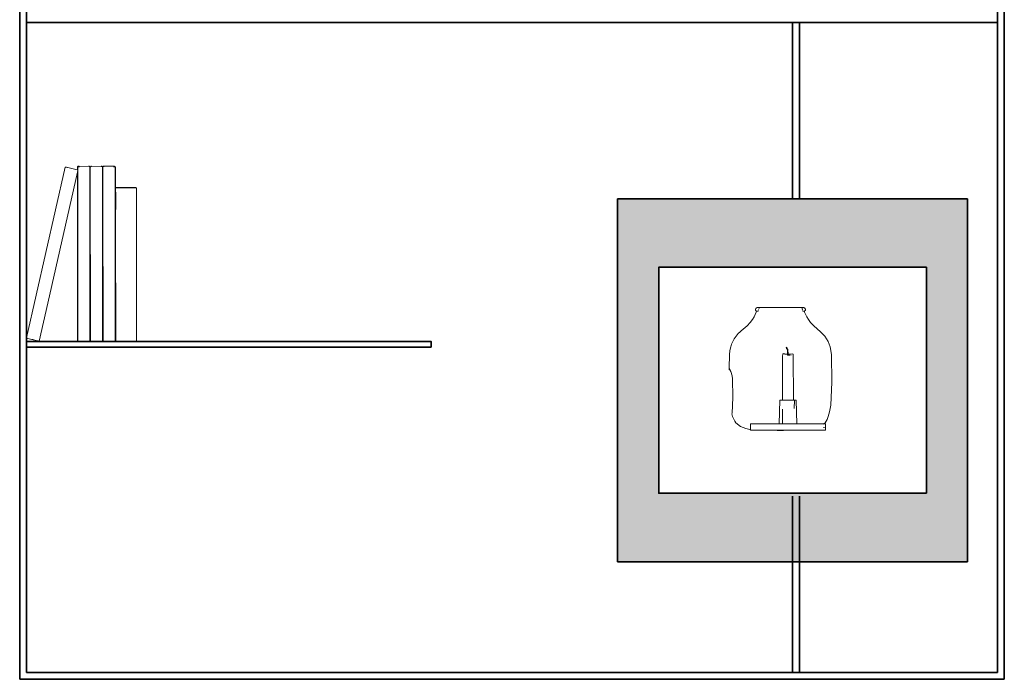
# Model space of a CAD drawing. Units: millimetres. Extents: x 2322 to 2394, y 1600 to 1790.
# Tile 1 of 5: x 2322 to 2394, y 1600 to 1648. Entities that reach past the tile are written whole.
import ezdxf

# ---------------------------------------------------------------- set-up
doc = ezdxf.new("R2010")
doc.units = ezdxf.units.MM
for name, color, linetype, lineweight in [('A-FURN', 7, 'Continuous', 35), ('A-FURN-ACCS', 8, 'Continuous', 18), ('A-FURN-PATT', 18, 'Continuous', 13)]:
    doc.layers.add(name, color=color, linetype=linetype, lineweight=lineweight)

msp = doc.modelspace()

# ---------------------------------------------------------------- hatches: boundary and pattern name
at = {"layer": 'A-FURN-PATT'}
h = msp.add_hatch(color=256, dxfattribs=at)
h.dxf.hatch_style = 1
h.paths.add_polyline_path([(2392.874, 1742.691), (2367.299, 1742.691), (2367.299, 1716.15), (2378.094, 1716.15), (2378.094, 1721.15), (2376.822, 1721.15), (2370.299, 1721.15), (2370.299, 1737.691), (2389.874, 1737.691), (2389.874, 1721.15), (2378.594, 1721.15), (2378.594, 1716.15), (2392.874, 1716.15)])
h.paths.add_polyline_path([(2352.154, 1685.571), (2339.867, 1685.571), (2339.867, 1680.571), (2349.154, 1680.571), (2349.154, 1664.029), (2329.579, 1664.029), (2329.579, 1680.571), (2339.367, 1680.571), (2339.367, 1685.571), (2326.579, 1685.571), (2326.579, 1659.029), (2352.154, 1659.029)])
h.paths.add_polyline_path([(2390.882, 1635.073), (2365.307, 1635.073), (2365.307, 1608.531), (2390.882, 1608.531)])
h.paths.add_polyline_path([(2387.882, 1630.073), (2387.882, 1613.531), (2368.307, 1613.531), (2368.307, 1630.073)], flags=16)
h.paths.add_polyline_path([(2373.463, 1622.711), (2373.46, 1622.644), (2373.462, 1622.642)], flags=0)
h.paths.add_polyline_path([(2380.387, 1618.619), (2380.387, 1618.619), (2380.35, 1618.619)], flags=0)
h.paths.add_polyline_path([(2377.431, 1618.132), (2377.363, 1618.141), (2377.19, 1618.152), (2377.145, 1618.149), (2376.982, 1618.132)], flags=0)
h.paths.add_polyline_path([(2376.126, 1618.152), (2375.767, 1618.152), (2375.734, 1618.152), (2375.734, 1618.152), (2375.028, 1618.152), (2375.028, 1618.198), (2374.578, 1618.295), (2374.235, 1618.449), (2373.926, 1618.69), (2373.709, 1619.163), (2373.66, 1619.336), (2373.672, 1619.402), (2373.73, 1620.54), (2373.702, 1622.038), (2373.678, 1622.131), (2373.705, 1621.917), (2373.73, 1620.54), (2373.667, 1619.311), (2373.709, 1619.163), (2373.87, 1618.812), (2373.949, 1618.699), (2374.037, 1618.604), (2374.187, 1618.486), (2374.3, 1618.42), (2374.485, 1618.337), (2374.688, 1618.272), (2374.979, 1618.209), (2375.028, 1618.203), (2375.028, 1618.372), (2375.028, 1618.619), (2377.125, 1618.619), (2377.165, 1620.356), (2377.172, 1620.356), (2377.172, 1620.357), (2377.341, 1620.357), (2377.354, 1620.357), (2377.354, 1623.532), (2377.38, 1623.766), (2377.629, 1623.72), (2377.726, 1623.72), (2377.722, 1623.891), (2377.719, 1624.041), (2377.644, 1624.123), (2377.631, 1624.228), (2377.644, 1624.211), (2377.677, 1624.213), (2377.688, 1624.153), (2377.757, 1624.059), (2377.78, 1623.72), (2377.883, 1623.72), (2378.152, 1623.76), (2378.155, 1620.358), (2378.298, 1620.356), (2378.301, 1620.356), (2378.362, 1620.357), (2378.402, 1618.619), (2377.354, 1618.619), (2377.125, 1618.619), (2375.028, 1618.619), (2375.028, 1618.372), (2375.028, 1618.177), (2375.049, 1618.152), (2375.734, 1618.152), (2375.756, 1618.153), (2375.767, 1618.152), (2376.126, 1618.152), (2376.144, 1618.154), (2376.168, 1618.151)], flags=0)
h.paths.add_polyline_path([(2380.5, 1618.343), (2380.401, 1618.342), (2380.5, 1618.342)], flags=0)
h.paths.add_polyline_path([(2378.836, 1627.111), (2378.86, 1627.114), (2378.771, 1627.114), (2378.773, 1627.108)], flags=0)
h.paths.add_polyline_path([(2378.972, 1627.091), (2379.09, 1626.957), (2378.972, 1626.879), (2378.964, 1626.862), (2378.975, 1626.787), (2379.128, 1626.434), (2379.25, 1626.246), (2379.42, 1626.03), (2379.646, 1625.791), (2380.15, 1625.354), (2380.519, 1624.956), (2380.743, 1624.553), (2380.884, 1624.119), (2380.94, 1623.673), (2380.977, 1621.652), (2380.892, 1619.98), (2380.807, 1619.502), (2380.712, 1619.163), (2380.621, 1618.942), (2380.422, 1618.619), (2380.413, 1618.619), (2380.386, 1618.619), (2380.474, 1618.703), (2380.621, 1618.942), (2380.712, 1619.163), (2380.807, 1619.502), (2380.892, 1619.98), (2380.977, 1621.652), (2380.94, 1623.673), (2380.9, 1623.987), (2380.843, 1624.244), (2380.778, 1624.446), (2380.693, 1624.644), (2380.585, 1624.839), (2380.452, 1625.029), (2380.15, 1625.354), (2379.646, 1625.791), (2379.324, 1626.132), (2379.128, 1626.434), (2378.92, 1626.915), (2378.841, 1626.975), (2378.869, 1626.811), (2379.027, 1626.915), (2379.041, 1626.939), (2379.037, 1626.997), (2379.02, 1627.036), (2378.879, 1627.196), (2378.841, 1627.151)], flags=0)
h.paths.add_polyline_path([(2375.501, 1627.114), (2375.642, 1627.103), (2375.561, 1626.855), (2375.555, 1626.827), (2375.48, 1626.868), (2375.292, 1626.434), (2375.097, 1626.132), (2374.775, 1625.791), (2374.271, 1625.354), (2374.13, 1625.216), (2373.969, 1625.029), (2373.836, 1624.839), (2373.728, 1624.644), (2373.643, 1624.446), (2373.537, 1624.119), (2373.52, 1623.987), (2373.601, 1624.348), (2373.773, 1624.748), (2374.034, 1625.122), (2374.271, 1625.354), (2374.775, 1625.791), (2375.001, 1626.03), (2375.171, 1626.246), (2375.292, 1626.434), (2375.445, 1626.787), (2375.447, 1626.797), (2375.334, 1627.042)], flags=0)
h.paths.add_polyline_path([(2375.398, 1627.114), (2375.384, 1626.997), (2375.411, 1627.054), (2375.531, 1627.169), (2375.597, 1627.114)], flags=0)
h.paths.add_polyline_path([(2377.985, 1623.628), (2377.785, 1623.645), (2377.786, 1623.634), (2377.764, 1623.634), (2377.729, 1623.636), (2377.728, 1623.656), (2377.701, 1623.664), (2377.421, 1623.752), (2377.412, 1623.748), (2377.629, 1623.72), (2377.78, 1623.72), (2377.783, 1623.68)], flags=0)
h.paths.add_polyline_path([(2377.348, 1620.356), (2377.335, 1620.356), (2377.327, 1620.356), (2377.354, 1620.356)], flags=0)
h.paths.add_polyline_path([(2377.834, 1620.357), (2377.854, 1620.356), (2377.911, 1620.356), (2377.923, 1620.357)], flags=0)
h.paths.add_polyline_path([(2378.155, 1620.356), (2378.155, 1620.356), (2378.014, 1620.356), (2378.002, 1620.357), (2377.96, 1620.356), (2377.956, 1620.356), (2377.923, 1620.357), (2378.111, 1620.357), (2378.119, 1620.356), (2378.144, 1620.356), (2378.163, 1620.357), (2378.163, 1620.357), (2378.157, 1620.357), (2378.149, 1620.356)], flags=0)
h.paths.add_polyline_path([(2377.609, 1620.357), (2377.623, 1620.356), (2377.653, 1620.357), (2377.738, 1620.356), (2377.743, 1620.357)], flags=0)
h.paths.add_polyline_path([(2380.479, 1618.152), (2380.406, 1618.152), (2380.313, 1618.151), (2380.107, 1618.152), (2380.104, 1618.152), (2380.108, 1618.151), (2379.961, 1618.152), (2379.793, 1618.152), (2377.32, 1618.152), (2377.3, 1618.149), (2377.253, 1618.152), (2379.793, 1618.152), (2380.01, 1618.153), (2380.21, 1618.152), (2380.229, 1618.152), (2380.231, 1618.152), (2380.394, 1618.152), (2380.48, 1618.152)], flags=0)

# ---------------------------------------------------------------- linework, layer by layer
at = {"layer": 'A-FURN'}
for p, q in [((2321.58, 1599.925), (2321.58, 1755.925)), ((2322.08, 1600.425), (2322.08, 1755.425)), ((2393.08, 1755.425), (2393.08, 1600.425)), ((2393.58, 1755.925), (2393.58, 1599.925)), ((2393.08, 1695.937), (2393.08, 1600.425)), ((2393.08, 1647.981), (2322.08, 1647.981)), ((2322.08, 1647.981), (2322.08, 1600.425)), ((2378.094, 1635.073), (2378.094, 1647.981)), ((2378.594, 1635.073), (2378.594, 1647.981)), ((2390.882, 1635.073), (2390.882, 1608.531)), ((2378.094, 1600.425), (2378.094, 1613.334)), ((2378.594, 1600.425), (2378.594, 1613.334)), ((2393.58, 1599.925), (2321.58, 1599.925)), ((2393.08, 1600.425), (2322.08, 1600.425))]:
    msp.add_line(p, q, dxfattribs=at)
for points in [[(2390.882, 1608.531), (2365.307, 1608.531), (2365.307, 1635.073), (2390.882, 1635.073)], [(2322.08, 1624.628), (2347.625, 1624.628), (2351.673, 1624.628), (2351.673, 1624.228)], [(2322.08, 1624.228), (2347.625, 1624.228), (2351.673, 1624.228)]]:
    msp.add_lwpolyline(points, dxfattribs=at)
msp.add_lwpolyline([(2387.882, 1613.531), (2368.307, 1613.531), (2368.307, 1630.073), (2387.882, 1630.073)], close=True, dxfattribs=at)
at = {"layer": 'A-FURN-ACCS'}
for p, q in [((2322.08, 1624.914), (2324.904, 1637.395)), ((2324.905, 1637.395), (2322.089, 1624.904)), ((2324.904, 1637.395), (2324.905, 1637.395)), ((2324.905, 1637.395), (2325.014, 1637.38)), ((2325.29, 1637.308), (2325.014, 1637.38)), ((2325.29, 1637.308), (2325.067, 1637.358)), ((2325.773, 1637.199), (2325.29, 1637.308)), ((2325.813, 1637.444), (2325.798, 1637.401)), ((2325.798, 1637.401), (2325.798, 1637.202)), ((2325.813, 1637.409), (2325.813, 1637.444)), ((2325.813, 1637.444), (2325.822, 1637.444)), ((2325.822, 1637.444), (2325.826, 1637.446)), ((2325.822, 1637.444), (2325.822, 1637.191)), ((2325.826, 1637.446), (2325.847, 1637.458)), ((2325.826, 1637.446), (2325.86, 1637.451)), ((2325.839, 1637.444), (2325.826, 1637.446)), ((2325.864, 1637.449), (2325.839, 1637.444)), ((2325.875, 1637.444), (2325.839, 1637.444)), ((2325.903, 1637.458), (2325.847, 1637.458)), ((2325.86, 1637.451), (2325.847, 1637.458)), ((2325.86, 1637.451), (2325.862, 1637.452)), ((2325.862, 1637.452), (2325.903, 1637.458)), ((2325.864, 1637.449), (2325.862, 1637.452)), ((2325.866, 1637.45), (2325.864, 1637.449)), ((2325.903, 1637.458), (2325.866, 1637.45)), ((2325.874, 1637.444), (2325.866, 1637.45)), ((2325.875, 1637.444), (2325.874, 1637.444)), ((2325.877, 1637.402), (2325.875, 1637.444)), ((2325.878, 1637.444), (2325.875, 1637.444)), ((2325.877, 1637.444), (2325.875, 1637.444)), ((2325.877, 1637.402), (2325.877, 1637.444)), ((2325.878, 1637.444), (2325.877, 1637.444)), ((2325.878, 1637.444), (2325.903, 1637.458)), ((2325.901, 1637.445), (2325.878, 1637.444)), ((2325.901, 1637.445), (2325.9, 1637.403)), ((2325.903, 1637.458), (2325.901, 1637.445)), ((2325.901, 1637.445), (2325.902, 1637.403)), ((2325.904, 1637.445), (2325.901, 1637.445)), ((2325.926, 1637.445), (2325.903, 1637.458)), ((2325.903, 1637.458), (2325.904, 1637.445)), ((2325.904, 1637.445), (2325.905, 1637.403)), ((2325.926, 1637.445), (2325.904, 1637.445)), ((2325.929, 1637.444), (2325.926, 1637.445)), ((2326.62, 1637.457), (2325.929, 1637.444)), ((2325.929, 1637.444), (2325.93, 1637.404)), ((2326.6, 1637.441), (2326.6, 1637.444)), ((2326.622, 1637.458), (2326.62, 1637.457)), ((2326.624, 1637.457), (2326.62, 1637.457)), ((2326.621, 1637.442), (2326.621, 1637.444)), ((2326.622, 1637.458), (2326.624, 1637.457)), ((2326.624, 1637.457), (2326.678, 1637.458)), ((2326.625, 1637.442), (2326.625, 1637.444)), ((2326.658, 1637.444), (2326.687, 1637.444)), ((2326.684, 1637.448), (2326.668, 1637.45)), ((2326.684, 1637.448), (2326.678, 1637.458)), ((2326.708, 1637.444), (2326.684, 1637.448)), ((2326.687, 1637.444), (2326.684, 1637.448)), ((2326.687, 1637.444), (2326.708, 1637.444)), ((2326.712, 1637.401), (2326.687, 1637.444)), ((2326.712, 1637.444), (2326.708, 1637.444)), ((2326.708, 1637.444), (2326.727, 1637.401)), ((2326.71, 1624.631), (2326.712, 1637.401)), ((2326.727, 1637.401), (2326.712, 1637.444)), ((2326.727, 1637.401), (2326.712, 1624.637)), ((2326.727, 1637.401), (2326.746, 1637.444)), ((2326.727, 1624.671), (2326.727, 1637.401)), ((2326.746, 1624.628), (2326.727, 1637.401)), ((2326.742, 1624.628), (2326.727, 1637.401)), ((2326.742, 1637.401), (2326.747, 1637.409)), ((2326.75, 1624.628), (2326.742, 1637.401)), ((2326.774, 1637.448), (2326.746, 1637.444)), ((2326.747, 1637.409), (2326.746, 1637.409)), ((2326.747, 1637.409), (2326.767, 1637.444)), ((2326.774, 1637.448), (2326.767, 1637.444)), ((2326.788, 1637.458), (2326.774, 1637.448)), ((2326.794, 1637.452), (2326.774, 1637.448)), ((2326.788, 1637.458), (2326.794, 1637.452)), ((2326.831, 1637.457), (2326.788, 1637.458)), ((2326.804, 1637.453), (2326.794, 1637.452)), ((2326.794, 1637.452), (2326.802, 1637.444)), ((2326.802, 1637.444), (2326.806, 1637.444)), ((2326.806, 1637.444), (2326.816, 1637.45)), ((2326.806, 1637.444), (2326.829, 1637.444)), ((2326.829, 1637.444), (2326.83, 1637.446)), ((2326.836, 1637.444), (2326.829, 1637.444)), ((2326.831, 1637.457), (2326.832, 1637.458)), ((2326.832, 1637.458), (2326.834, 1637.457)), ((2327.54, 1637.445), (2326.834, 1637.457)), ((2327.54, 1637.445), (2327.548, 1637.458)), ((2327.554, 1637.444), (2327.54, 1637.445)), ((2327.548, 1637.458), (2327.611, 1637.458)), ((2327.553, 1637.447), (2327.554, 1637.444)), ((2327.587, 1637.444), (2327.554, 1637.444)), ((2327.616, 1637.444), (2327.579, 1637.452)), ((2327.616, 1637.444), (2327.611, 1637.458)), ((2327.622, 1637.438), (2327.616, 1637.444)), ((2327.641, 1637.401), (2327.622, 1637.438)), ((2327.656, 1637.401), (2327.622, 1637.438)), ((2327.641, 1627.214), (2327.656, 1637.401)), ((2327.656, 1637.401), (2327.641, 1624.671)), ((2327.641, 1627.214), (2327.641, 1637.401)), ((2327.656, 1624.671), (2327.671, 1637.401)), ((2327.671, 1637.401), (2327.67, 1637.444)), ((2327.67, 1637.444), (2327.673, 1637.444)), ((2327.671, 1637.401), (2327.673, 1637.444)), ((2327.671, 1637.401), (2327.672, 1635.669)), ((2327.706, 1637.458), (2327.673, 1637.444)), ((2327.673, 1637.444), (2327.675, 1637.444)), ((2327.716, 1637.451), (2327.675, 1637.444)), ((2327.706, 1637.458), (2328.524, 1637.458)), ((2327.735, 1637.444), (2327.758, 1637.444)), ((2327.758, 1637.444), (2327.758, 1637.442)), ((2327.762, 1637.442), (2327.762, 1637.444)), ((2327.78, 1637.444), (2327.786, 1637.444)), ((2327.786, 1637.44), (2327.786, 1637.444)), ((2328.468, 1637.444), (2328.465, 1637.404)), ((2328.483, 1637.444), (2328.477, 1637.403)), ((2328.483, 1637.444), (2328.481, 1637.403)), ((2328.483, 1637.403), (2328.483, 1637.444)), ((2328.506, 1637.402), (2328.506, 1637.444)), ((2328.509, 1637.401), (2328.51, 1637.444)), ((2328.554, 1637.446), (2328.524, 1637.458)), ((2328.537, 1637.449), (2328.539, 1637.448)), ((2328.539, 1637.448), (2328.554, 1637.446)), ((2328.554, 1637.446), (2328.544, 1637.444)), ((2328.561, 1637.444), (2328.554, 1637.446)), ((2328.561, 1637.444), (2328.562, 1624.628)), ((2328.566, 1637.444), (2328.561, 1637.444)), ((2328.57, 1637.444), (2328.566, 1637.444)), ((2328.566, 1637.444), (2328.57, 1637.434)), ((2328.585, 1637.401), (2328.57, 1637.444)), ((2328.57, 1637.444), (2328.57, 1637.434)), ((2328.57, 1637.434), (2328.57, 1637.409)), ((2328.57, 1637.434), (2328.585, 1637.401)), ((2328.585, 1624.671), (2328.585, 1637.401)), ((2325.797, 1637.027), (2323.637, 1627.451)), ((2325.792, 1637.205), (2325.773, 1637.199)), ((2325.773, 1637.199), (2325.822, 1637.188)), ((2325.792, 1637.205), (2325.798, 1637.202)), ((2325.797, 1637.027), (2325.822, 1637.139)), ((2325.797, 1637.027), (2325.798, 1624.671)), ((2325.822, 1637.191), (2325.798, 1637.202)), ((2325.798, 1637.202), (2325.798, 1637.197)), ((2325.822, 1637.139), (2325.821, 1624.628)), ((2325.831, 1637.186), (2325.822, 1637.191)), ((2325.822, 1637.191), (2325.822, 1637.188)), ((2325.831, 1637.186), (2325.822, 1637.188)), ((2325.822, 1637.146), (2325.831, 1637.186)), ((2325.822, 1637.146), (2325.822, 1637.139)), ((2328.585, 1624.671), (2328.597, 1635.853)), ((2328.596, 1635.889), (2328.6, 1635.889)), ((2328.597, 1635.853), (2328.596, 1635.889)), ((2328.597, 1635.853), (2328.6, 1635.889)), ((2328.597, 1635.853), (2328.599, 1635.297)), ((2328.632, 1635.901), (2328.6, 1635.889)), ((2328.639, 1635.889), (2328.6, 1635.889)), ((2328.632, 1635.901), (2328.643, 1635.889)), ((2330.048, 1635.901), (2328.632, 1635.901)), ((2328.665, 1635.889), (2328.632, 1635.901)), ((2328.643, 1635.889), (2328.639, 1635.889)), ((2328.646, 1635.889), (2328.643, 1635.889)), ((2328.643, 1635.889), (2328.645, 1635.889)), ((2328.645, 1635.889), (2328.646, 1635.889)), ((2328.665, 1635.889), (2328.646, 1635.889)), ((2328.665, 1635.889), (2328.676, 1635.889)), ((2328.676, 1635.889), (2328.679, 1635.889)), ((2328.679, 1635.889), (2330.031, 1635.889)), ((2330.031, 1635.889), (2330.048, 1635.901)), ((2330.05, 1635.899), (2330.031, 1635.889)), ((2330.031, 1635.889), (2330.05, 1635.889)), ((2330.048, 1635.901), (2330.05, 1635.901)), ((2330.05, 1635.899), (2330.05, 1635.901)), ((2330.085, 1635.901), (2330.05, 1635.901)), ((2330.08, 1635.896), (2330.05, 1635.901)), ((2330.05, 1635.889), (2330.05, 1635.899)), ((2330.053, 1635.889), (2330.05, 1635.899)), ((2330.058, 1635.889), (2330.05, 1635.899)), ((2330.053, 1635.889), (2330.05, 1635.889)), ((2330.053, 1635.889), (2330.058, 1635.889)), ((2330.074, 1635.889), (2330.058, 1635.889)), ((2330.074, 1635.889), (2330.08, 1635.896)), ((2330.074, 1635.889), (2330.11, 1635.891)), ((2330.08, 1635.896), (2330.085, 1635.901)), ((2330.11, 1635.891), (2330.08, 1635.896)), ((2330.11, 1635.891), (2330.085, 1635.901)), ((2330.115, 1635.889), (2330.11, 1635.891)), ((2330.115, 1624.628), (2330.115, 1635.889)), ((2330.118, 1635.889), (2330.115, 1635.889)), ((2330.121, 1635.889), (2330.118, 1635.889)), ((2330.118, 1635.889), (2330.121, 1635.881)), ((2330.133, 1635.853), (2330.121, 1635.889)), ((2330.121, 1635.889), (2330.121, 1635.881)), ((2330.121, 1635.881), (2330.121, 1635.859)), ((2330.121, 1635.881), (2330.133, 1635.853)), ((2330.133, 1624.662), (2330.133, 1635.853)), ((2327.672, 1635.669), (2327.656, 1624.671)), ((2327.672, 1635.669), (2327.679, 1624.628)), ((2328.599, 1635.297), (2328.596, 1633.242)), ((2328.596, 1633.242), (2328.585, 1624.671)), ((2328.596, 1624.635), (2328.596, 1633.242)), ((2328.596, 1633.242), (2328.603, 1624.628)), ((2323.011, 1624.674), (2323.637, 1627.451)), ((2323.637, 1627.451), (2323.013, 1624.674)), ((2327.641, 1624.671), (2327.641, 1627.214)), ((2375.292, 1626.434), (2375.445, 1626.787)), ((2375.378, 1626.947), (2375.384, 1626.997)), ((2375.378, 1626.947), (2375.391, 1626.918)), ((2375.384, 1626.997), (2375.411, 1627.054)), ((2375.435, 1626.893), (2375.391, 1626.918)), ((2375.411, 1627.054), (2375.453, 1627.094)), ((2375.457, 1626.862), (2375.435, 1626.893)), ((2375.445, 1626.787), (2375.457, 1626.862)), ((2375.453, 1627.094), (2375.501, 1627.114)), ((2375.501, 1627.114), (2375.608, 1627.106)), ((2375.501, 1627.114), (2376.761, 1627.114)), ((2375.561, 1626.855), (2375.551, 1626.805)), ((2375.576, 1626.901), (2375.561, 1626.855)), ((2375.602, 1626.979), (2375.585, 1626.929)), ((2375.608, 1627.106), (2375.647, 1627.074)), ((2375.647, 1627.074), (2375.65, 1627.055)), ((2376.774, 1627.114), (2376.761, 1627.114)), ((2376.774, 1627.114), (2378.86, 1627.114)), ((2378.768, 1627.108), (2378.836, 1627.111)), ((2378.793, 1627.096), (2378.774, 1627.075)), ((2378.785, 1627.017), (2378.812, 1626.997)), ((2378.836, 1627.111), (2378.793, 1627.096)), ((2378.812, 1626.997), (2378.818, 1626.978)), ((2378.834, 1626.934), (2378.837, 1626.925)), ((2378.86, 1627.114), (2378.836, 1627.111)), ((2378.842, 1626.91), (2378.861, 1626.857)), ((2378.863, 1627.114), (2378.86, 1627.114)), ((2378.861, 1626.857), (2378.87, 1626.803)), ((2378.863, 1627.114), (2378.923, 1627.114)), ((2378.972, 1627.091), (2378.923, 1627.114)), ((2378.964, 1626.862), (2378.972, 1626.879)), ((2378.975, 1626.787), (2378.964, 1626.862)), ((2379.02, 1627.036), (2378.972, 1627.091)), ((2378.972, 1626.879), (2379.027, 1626.915)), ((2379.128, 1626.434), (2378.975, 1626.787)), ((2379.037, 1626.997), (2379.02, 1627.036)), ((2379.027, 1626.915), (2379.041, 1626.939)), ((2379.041, 1626.939), (2379.037, 1626.997)), ((2374.334, 1625.409), (2374.775, 1625.791)), ((2374.775, 1625.791), (2375.001, 1626.03)), ((2375.001, 1626.03), (2375.171, 1626.246)), ((2375.171, 1626.246), (2375.292, 1626.434)), ((2379.25, 1626.246), (2379.128, 1626.434)), ((2379.42, 1626.03), (2379.25, 1626.246)), ((2379.646, 1625.791), (2379.42, 1626.03)), ((2380.15, 1625.354), (2379.646, 1625.791)), ((2373.969, 1625.029), (2374.13, 1625.216)), ((2374.13, 1625.216), (2374.271, 1625.354)), ((2374.271, 1625.354), (2374.334, 1625.409)), ((2380.452, 1625.029), (2380.15, 1625.354)), ((2322.08, 1624.914), (2322.084, 1624.883)), ((2322.084, 1624.883), (2322.089, 1624.904)), ((2322.084, 1624.883), (2322.086, 1624.883)), ((2322.089, 1624.904), (2322.086, 1624.883)), ((2322.181, 1624.862), (2322.086, 1624.883)), ((2322.181, 1624.862), (2322.471, 1624.786)), ((2322.471, 1624.786), (2322.549, 1624.779)), ((2322.996, 1624.668), (2322.471, 1624.786)), ((2322.692, 1624.746), (2322.549, 1624.779)), ((2322.692, 1624.746), (2322.695, 1624.745)), ((2322.996, 1624.668), (2322.961, 1624.684)), ((2322.996, 1624.668), (2322.997, 1624.678)), ((2322.996, 1624.668), (2323.011, 1624.674)), ((2323.013, 1624.674), (2323.011, 1624.674)), ((2325.798, 1624.671), (2325.813, 1624.628)), ((2325.813, 1624.637), (2325.798, 1624.671)), ((2325.813, 1624.628), (2325.813, 1624.637)), ((2325.817, 1624.628), (2325.813, 1624.637)), ((2325.813, 1624.628), (2325.817, 1624.628)), ((2325.821, 1624.628), (2325.817, 1624.628)), ((2325.821, 1624.628), (2326.71, 1624.628)), ((2326.712, 1624.637), (2326.71, 1624.631)), ((2326.71, 1624.628), (2326.71, 1624.631)), ((2326.71, 1624.628), (2326.712, 1624.628)), ((2326.712, 1624.628), (2326.727, 1624.671)), ((2326.727, 1624.671), (2326.712, 1624.637)), ((2326.712, 1624.637), (2326.712, 1624.628)), ((2326.742, 1624.628), (2326.712, 1624.628)), ((2326.746, 1624.628), (2326.742, 1624.628)), ((2326.746, 1624.628), (2326.75, 1624.628)), ((2327.633, 1624.628), (2326.75, 1624.628)), ((2327.637, 1624.651), (2327.633, 1624.628)), ((2327.637, 1624.628), (2327.633, 1624.628)), ((2327.641, 1624.671), (2327.637, 1624.651)), ((2327.637, 1624.628), (2327.637, 1624.651)), ((2327.641, 1624.628), (2327.637, 1624.628)), ((2327.641, 1624.671), (2327.641, 1624.628)), ((2327.67, 1624.628), (2327.641, 1624.628)), ((2327.656, 1624.671), (2327.67, 1624.628)), ((2327.67, 1624.637), (2327.656, 1624.671)), ((2327.67, 1624.628), (2327.67, 1624.637)), ((2327.675, 1624.628), (2327.67, 1624.637)), ((2327.67, 1624.628), (2327.675, 1624.628)), ((2327.679, 1624.628), (2327.675, 1624.628)), ((2327.679, 1624.628), (2328.562, 1624.628)), ((2328.566, 1624.628), (2328.562, 1624.628)), ((2328.57, 1624.637), (2328.566, 1624.628)), ((2328.566, 1624.628), (2328.57, 1624.628)), ((2328.57, 1624.628), (2328.585, 1624.671)), ((2328.585, 1624.671), (2328.57, 1624.637)), ((2328.57, 1624.663), (2328.57, 1624.637)), ((2328.57, 1624.637), (2328.57, 1624.628)), ((2328.596, 1624.628), (2328.57, 1624.628)), ((2328.585, 1624.662), (2328.585, 1624.671)), ((2328.585, 1624.662), (2328.596, 1624.628)), ((2328.596, 1624.635), (2328.585, 1624.662)), ((2328.596, 1624.628), (2328.596, 1624.635)), ((2328.599, 1624.628), (2328.596, 1624.635)), ((2328.599, 1624.628), (2328.596, 1624.628)), ((2328.603, 1624.628), (2328.599, 1624.628)), ((2330.115, 1624.628), (2328.603, 1624.628)), ((2330.119, 1624.628), (2330.115, 1624.628)), ((2330.121, 1624.634), (2330.119, 1624.628)), ((2330.122, 1624.628), (2330.119, 1624.628)), ((2330.133, 1624.662), (2330.121, 1624.634)), ((2330.121, 1624.634), (2330.122, 1624.628)), ((2330.122, 1624.628), (2330.133, 1624.662)), ((2373.578, 1624.244), (2373.643, 1624.446)), ((2373.643, 1624.446), (2373.728, 1624.644)), ((2373.836, 1624.839), (2373.728, 1624.644)), ((2373.969, 1625.029), (2373.836, 1624.839)), ((2380.585, 1624.839), (2380.452, 1625.029)), ((2380.693, 1624.644), (2380.585, 1624.839)), ((2380.778, 1624.446), (2380.693, 1624.644)), ((2380.843, 1624.244), (2380.778, 1624.446)), ((2373.463, 1622.711), (2373.481, 1623.673)), ((2373.481, 1623.673), (2373.52, 1623.987)), ((2373.52, 1623.987), (2373.578, 1624.244)), ((2377.354, 1623.532), (2377.376, 1623.731)), ((2377.431, 1623.757), (2377.376, 1623.731)), ((2377.629, 1623.72), (2377.431, 1623.757)), ((2377.589, 1623.699), (2377.449, 1623.743)), ((2377.449, 1623.743), (2377.629, 1623.72)), ((2377.629, 1623.72), (2377.726, 1623.72)), ((2377.727, 1623.694), (2377.629, 1623.72)), ((2377.677, 1624.213), (2377.633, 1624.21)), ((2377.644, 1624.123), (2377.633, 1624.21)), ((2377.719, 1624.041), (2377.644, 1624.123)), ((2377.688, 1624.153), (2377.677, 1624.213)), ((2377.757, 1624.059), (2377.688, 1624.153)), ((2377.728, 1623.656), (2377.701, 1623.664)), ((2377.722, 1623.891), (2377.719, 1624.041)), ((2377.726, 1623.72), (2377.722, 1623.891)), ((2377.727, 1623.694), (2377.726, 1623.72)), ((2377.726, 1623.72), (2377.78, 1623.72)), ((2377.783, 1623.68), (2377.727, 1623.694)), ((2377.727, 1623.685), (2377.727, 1623.69)), ((2377.728, 1623.656), (2377.728, 1623.673)), ((2377.756, 1623.647), (2377.728, 1623.656)), ((2377.729, 1623.636), (2377.728, 1623.656)), ((2377.764, 1623.634), (2377.729, 1623.636)), ((2377.756, 1623.647), (2377.785, 1623.645)), ((2377.757, 1624.059), (2377.78, 1623.72)), ((2377.764, 1623.634), (2377.786, 1623.634)), ((2377.78, 1623.72), (2377.783, 1623.68)), ((2377.78, 1623.72), (2377.883, 1623.72)), ((2377.985, 1623.628), (2377.783, 1623.68)), ((2377.783, 1623.673), (2377.784, 1623.655)), ((2377.785, 1623.645), (2377.786, 1623.634)), ((2377.785, 1623.645), (2377.889, 1623.636)), ((2377.883, 1623.72), (2378.062, 1623.747)), ((2378.062, 1623.747), (2378.135, 1623.719)), ((2378.152, 1623.654), (2378.135, 1623.719)), ((2378.152, 1623.654), (2378.155, 1620.356)), ((2380.9, 1623.987), (2380.843, 1624.244)), ((2380.94, 1623.673), (2380.9, 1623.987)), ((2380.977, 1621.652), (2380.94, 1623.673)), ((2377.354, 1620.356), (2377.354, 1623.532)), ((2373.46, 1622.644), (2373.463, 1622.711)), ((2373.462, 1622.642), (2373.46, 1622.644)), ((2373.461, 1622.571), (2373.462, 1622.642)), ((2373.512, 1622.56), (2373.462, 1622.642)), ((2373.463, 1622.711), (2373.594, 1622.443)), ((2373.555, 1622.443), (2373.512, 1622.56)), ((2373.594, 1622.443), (2373.678, 1622.131)), ((2373.678, 1622.131), (2373.705, 1621.917)), ((2373.705, 1621.917), (2373.73, 1620.54)), ((2380.892, 1619.98), (2380.977, 1621.652)), ((2373.73, 1620.54), (2373.672, 1619.402)), ((2377.125, 1618.619), (2377.165, 1620.351)), ((2377.165, 1620.351), (2377.172, 1620.356)), ((2377.172, 1620.356), (2377.224, 1620.356)), ((2377.224, 1620.356), (2377.227, 1620.356)), ((2377.227, 1620.356), (2377.25, 1620.356)), ((2377.25, 1620.356), (2377.255, 1620.356)), ((2377.255, 1620.356), (2377.257, 1620.356)), ((2377.257, 1620.356), (2377.273, 1620.356)), ((2377.273, 1620.356), (2377.281, 1620.357)), ((2377.281, 1620.357), (2377.286, 1620.356)), ((2377.286, 1620.356), (2377.289, 1620.357)), ((2377.289, 1620.357), (2377.292, 1620.356)), ((2377.292, 1620.356), (2377.298, 1620.357)), ((2377.302, 1620.357), (2377.298, 1620.357)), ((2377.298, 1620.357), (2377.298, 1620.351)), ((2377.302, 1620.357), (2377.305, 1620.357)), ((2377.305, 1620.357), (2377.312, 1620.357)), ((2377.324, 1620.357), (2377.312, 1620.357)), ((2377.327, 1620.356), (2377.324, 1620.357)), ((2377.327, 1620.356), (2377.338, 1620.356)), ((2377.338, 1620.356), (2377.341, 1620.357)), ((2377.341, 1620.357), (2377.343, 1620.357)), ((2377.343, 1620.357), (2377.354, 1620.356)), ((2377.354, 1620.351), (2377.354, 1620.356)), ((2377.369, 1620.356), (2377.354, 1620.356)), ((2377.369, 1620.356), (2377.387, 1620.357)), ((2377.452, 1620.357), (2377.387, 1620.357)), ((2377.462, 1620.356), (2377.452, 1620.357)), ((2377.462, 1620.356), (2377.514, 1620.356)), ((2377.514, 1620.356), (2377.526, 1620.357)), ((2377.526, 1620.357), (2377.609, 1620.357)), ((2377.623, 1620.356), (2377.609, 1620.357)), ((2377.623, 1620.356), (2377.653, 1620.357)), ((2377.738, 1620.356), (2377.653, 1620.357)), ((2377.738, 1620.356), (2377.743, 1620.357)), ((2377.743, 1620.357), (2377.834, 1620.357)), ((2377.854, 1620.356), (2377.834, 1620.357)), ((2377.854, 1620.356), (2377.911, 1620.356)), ((2377.911, 1620.356), (2377.923, 1620.357)), ((2377.956, 1620.356), (2377.923, 1620.357)), ((2377.96, 1620.356), (2377.956, 1620.356)), ((2377.965, 1620.357), (2377.96, 1620.356)), ((2377.965, 1620.357), (2377.969, 1620.356)), ((2377.969, 1620.356), (2377.971, 1620.356)), ((2377.971, 1620.356), (2378.002, 1620.357)), ((2378.014, 1620.356), (2378.002, 1620.357)), ((2378.038, 1620.356), (2378.014, 1620.356)), ((2378.038, 1620.356), (2378.043, 1620.357)), ((2378.043, 1620.357), (2378.111, 1620.357)), ((2378.119, 1620.356), (2378.111, 1620.357)), ((2378.119, 1620.356), (2378.144, 1620.356)), ((2378.15, 1620.356), (2378.144, 1620.356)), ((2378.155, 1620.356), (2378.15, 1620.356)), ((2378.157, 1620.357), (2378.155, 1620.356)), ((2378.155, 1620.356), (2378.155, 1620.351)), ((2378.163, 1620.357), (2378.157, 1620.357)), ((2378.165, 1620.357), (2378.163, 1620.357)), ((2378.165, 1620.357), (2378.178, 1620.356)), ((2378.183, 1620.356), (2378.178, 1620.356)), ((2378.2, 1620.356), (2378.183, 1620.356)), ((2378.205, 1620.356), (2378.2, 1620.356)), ((2378.205, 1620.356), (2378.217, 1620.357)), ((2378.23, 1620.357), (2378.217, 1620.357)), ((2378.23, 1620.357), (2378.221, 1619.743)), ((2378.234, 1620.357), (2378.23, 1620.357)), ((2378.238, 1620.356), (2378.234, 1620.357)), ((2378.238, 1620.356), (2378.262, 1620.356)), ((2378.262, 1620.356), (2378.268, 1620.356)), ((2378.268, 1620.356), (2378.274, 1620.356)), ((2378.274, 1620.356), (2378.294, 1620.356)), ((2378.294, 1620.356), (2378.298, 1620.356)), ((2378.298, 1620.356), (2378.301, 1620.356)), ((2378.301, 1620.356), (2378.31, 1620.356)), ((2378.31, 1620.356), (2378.356, 1620.356)), ((2378.362, 1620.351), (2378.356, 1620.356)), ((2378.402, 1618.619), (2378.362, 1620.351)), ((2373.672, 1619.402), (2373.66, 1619.336)), ((2373.709, 1619.163), (2373.66, 1619.336)), ((2377.354, 1618.619), (2377.354, 1619.68)), ((2380.712, 1619.163), (2380.807, 1619.502)), ((2380.807, 1619.502), (2380.892, 1619.98)), ((2373.87, 1618.812), (2373.709, 1619.163)), ((2373.949, 1618.699), (2373.87, 1618.812)), ((2374.037, 1618.604), (2373.949, 1618.699)), ((2374.187, 1618.486), (2374.037, 1618.604)), ((2375.028, 1618.372), (2375.028, 1618.619)), ((2377.125, 1618.619), (2375.028, 1618.619)), ((2377.354, 1618.619), (2377.125, 1618.619)), ((2377.354, 1618.619), (2378.402, 1618.619)), ((2380.35, 1618.619), (2378.402, 1618.619)), ((2380.35, 1618.583), (2380.387, 1618.619)), ((2380.35, 1618.619), (2380.387, 1618.619)), ((2380.387, 1618.619), (2380.472, 1618.699)), ((2380.398, 1618.619), (2380.387, 1618.619)), ((2380.413, 1618.619), (2380.398, 1618.619)), ((2380.413, 1618.619), (2380.499, 1618.619)), ((2380.472, 1618.699), (2380.621, 1618.942)), ((2380.5, 1618.177), (2380.499, 1618.619)), ((2380.621, 1618.942), (2380.712, 1619.163)), ((2374.3, 1618.42), (2374.187, 1618.486)), ((2374.485, 1618.337), (2374.3, 1618.42)), ((2374.688, 1618.272), (2374.485, 1618.337)), ((2374.979, 1618.209), (2374.688, 1618.272)), ((2375.028, 1618.203), (2374.979, 1618.209)), ((2375.028, 1618.203), (2375.028, 1618.372)), ((2375.028, 1618.177), (2375.028, 1618.203)), ((2375.049, 1618.152), (2375.028, 1618.177)), ((2375.734, 1618.152), (2375.049, 1618.152)), ((2375.756, 1618.153), (2375.734, 1618.152)), ((2375.767, 1618.152), (2375.756, 1618.153)), ((2375.767, 1618.152), (2376.126, 1618.152)), ((2376.126, 1618.152), (2375.956, 1618.153)), ((2376.144, 1618.154), (2376.126, 1618.152)), ((2376.164, 1618.152), (2376.144, 1618.154)), ((2376.164, 1618.152), (2377.137, 1618.152)), ((2376.982, 1618.132), (2377.145, 1618.149)), ((2376.982, 1618.132), (2377.431, 1618.132)), ((2377.145, 1618.149), (2377.137, 1618.152)), ((2377.145, 1618.149), (2377.19, 1618.152)), ((2377.235, 1618.149), (2377.19, 1618.152)), ((2377.253, 1618.152), (2377.235, 1618.149)), ((2377.253, 1618.152), (2377.3, 1618.149)), ((2377.3, 1618.149), (2377.32, 1618.152)), ((2377.431, 1618.132), (2377.3, 1618.149)), ((2377.32, 1618.152), (2379.793, 1618.152)), ((2379.793, 1618.152), (2379.961, 1618.152)), ((2380.082, 1618.152), (2379.961, 1618.152)), ((2380.082, 1618.152), (2380.104, 1618.152)), ((2380.104, 1618.152), (2380.105, 1618.152)), ((2380.104, 1618.152), (2380.107, 1618.152)), ((2380.107, 1618.152), (2380.21, 1618.152)), ((2380.21, 1618.152), (2380.229, 1618.152)), ((2380.229, 1618.152), (2380.231, 1618.152)), ((2380.231, 1618.152), (2380.314, 1618.152)), ((2380.314, 1618.152), (2380.371, 1618.152)), ((2380.401, 1618.342), (2380.35, 1618.342)), ((2380.371, 1618.152), (2380.394, 1618.152)), ((2380.406, 1618.152), (2380.394, 1618.152)), ((2380.426, 1618.342), (2380.401, 1618.342)), ((2380.479, 1618.152), (2380.406, 1618.152)), ((2380.479, 1618.152), (2380.5, 1618.177))]:
    msp.add_line(p, q, dxfattribs=at)

doc.saveas('drawing.dxf')
